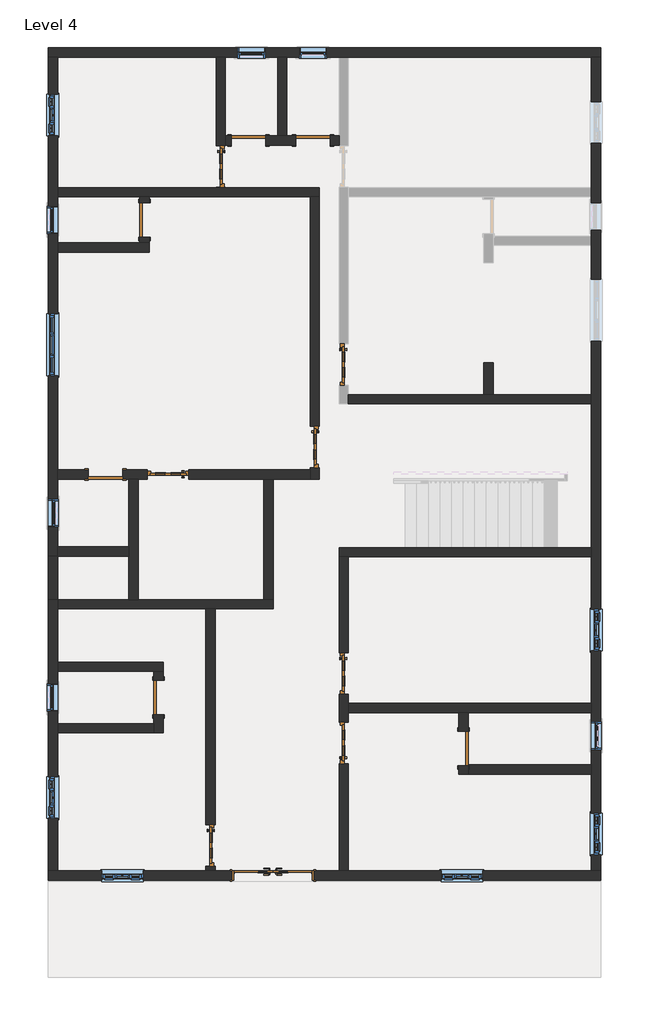
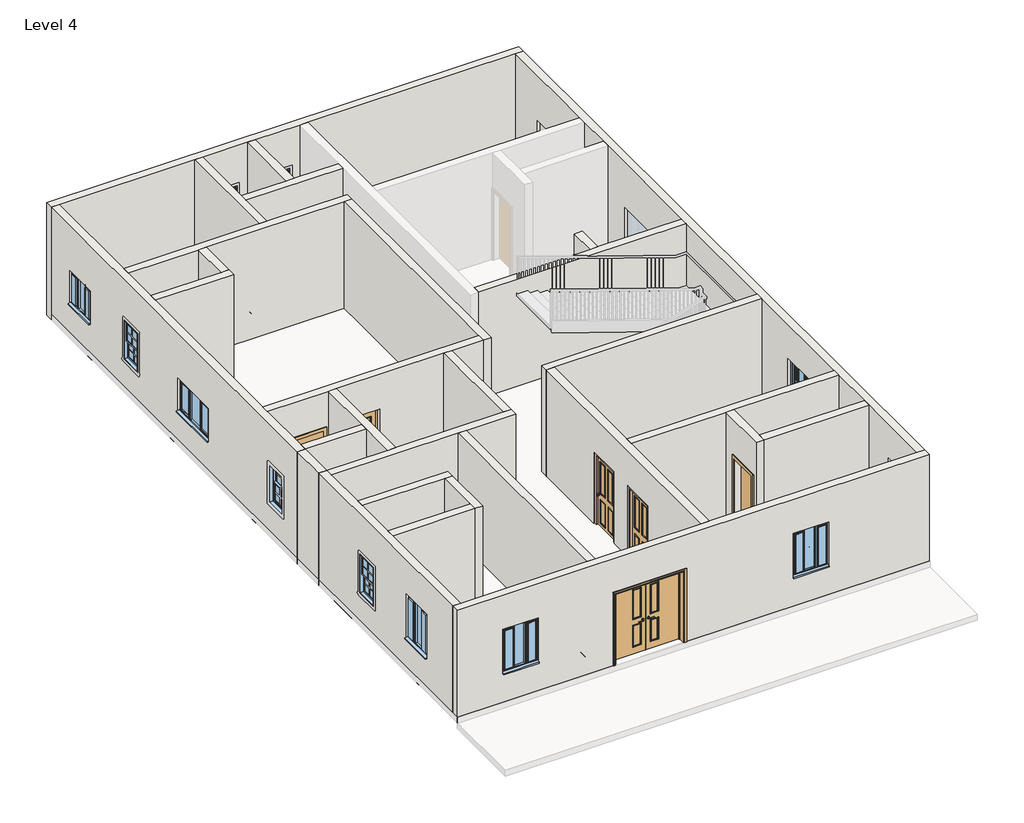
# One storey, part 1 of 3: 29 walls, 14 doors, 13 windows.
# Revit data of these elements (continued)
# Type "Windows_Tpl_Plain : 1360x910mm" (continued)
#   Cavity Closer Depth = 0' - 3.34646"
#   Vis - Cavity Closers = yes
#   Define Thermal Properties by = 1
#   Material Trim = Window Frame
#   Material Glass = Glass
#   Material Frame = Window Frame
#   Wall Closure = (empty or 0)
# Type "Windows_Tpl_w-Glazing_Cross-Bars : 910x1210mm"
#   Type Mark = "25"
#   Operation = "TriplePanelVertical"
#   Construction Type Id = "GSP4R"
#   Manufacturer = "Revit"
#   Keynote = "L10"
#   Analytic Construction = "1/8 in Pilkington single glazing"
#   Wrap Layers (Ext) from Ext = 0' - 4.03543"
#   Wrap Layers (Int) from Ext = 0' - 6.98819"
#   Window Board Projection = 0' - 0.98425"
#   Window Board Extension = 0' - 0.98425"
#   Visual Light Transmittance = 0.9
#   Solar Heat Gain Coefficient = 0.78
#   Rough Width = 2' - 11.82677"
#   Rough Height = 3' - 11.6378"
#   Height = 3' - 11.6378"
#   Width = 2' - 11.82677"
#   Heat Transfer Coefficient (U) = 0.6496 BTU/(h·ft²·°F)
#   Glazing Thickness = 0' - 0.94488"
#   Glazing Bar Thickness = 0' - 0.7874"
#   FrameOffset - External = 0' - 1.9685"
#   Frame Depth = 0' - 2.55906"
#   Default Head Height = 6' - 11.07087"
#   Cill Depth = 0' - 3.44488"
#   Cavity Closer Width = 0' - 1.9685"
#   Cavity Closer Offset from Ext = 0' - 4.03543"
#   Cavity Closer Depth = 0' - 3.34646"
#   Vis - Glazing Bars = yes
#   Vis - Cavity Closers = yes
#   Define Thermal Properties by = 1
#   Material Trim = Window Frame
#   Material Glazing Bars = Window Frame
#   Material Glass = Glass
#   Material Frame = Window Frame
#   Wall Closure = (empty or 0)
# Type "Windows_Tpl_w-Glazing_Cross-Bars : 910x910mm"
#   Type Mark = "24"
#   Operation = "TriplePanelVertical"
#   Construction Type Id = "GSP4R"
#   Manufacturer = "Revit"
#   Keynote = "L10"
#   Analytic Construction = "1/8 in Pilkington single glazing"
#   Wrap Layers (Ext) from Ext = 0' - 4.03543"
#   Wrap Layers (Int) from Ext = 0' - 6.98819"
#   Window Board Projection = 0' - 0.98425"
#   Window Board Extension = 0' - 0.98425"
#   Visual Light Transmittance = 0.9
#   Solar Heat Gain Coefficient = 0.78
#   Rough Width = 2' - 11.82677"
#   Rough Height = 2' - 11.82677"
#   Height = 2' - 11.82677"
#   Width = 2' - 11.82677"
#   Heat Transfer Coefficient (U) = 0.6496 BTU/(h·ft²·°F)
#   Glazing Thickness = 0' - 0.94488"
#   Glazing Bar Thickness = 0' - 0.7874"
#   FrameOffset - External = 0' - 1.9685"
#   Frame Depth = 0' - 2.55906"
#   Default Head Height = 6' - 11.07087"
#   Cill Depth = 0' - 3.44488"
#   Cavity Closer Width = 0' - 1.9685"
#   Cavity Closer Offset from Ext = 0' - 4.03543"
#   Cavity Closer Depth = 0' - 3.34646"
#   Vis - Glazing Bars = yes
#   Vis - Cavity Closers = yes
#   Define Thermal Properties by = 1
#   Material Trim = Window Frame
#   Material Glazing Bars = Window Frame
#   Material Glass = Glass
#   Material Frame = Window Frame
#   Wall Closure = (empty or 0)
# Elements 1, 2, 3, 4, 5, 6, 7 (IfcDoor, "Doors_ExtSgl_2 : 2'x7\"")
#   Phase Created = New Construction
#   Materials on its faces: "Door - Panel", "Door - Handle", "Door - Frame/Mullion", "Door - Glazing"
# Element 8 (IfcDoor, "Doors_IntDbl_3 : 1810x2110mm")
#   Phase Created = New Construction
#   Materials on its faces: "Door - Panel", "Door - Handle", "Door - Architrave", "Door - Frame/Mullion", "Door - Glazing"
# Elements 9, 10, 11, 12, 13, 14 (IfcDoor, "Single-Flush : 30\" x 80\"")
#   Phase Created = New Construction
#   Materials on its faces: "Door - Frame", "Door - Panel"
# Elements 15, 16, 17, 18, 19, 20, 21, 22, 23, 24, 25, 26, 27, 28, 29, 30, 31, 32, 34, 35, 36, 37 (IfcWall, "Generic - 4.5\" p")
#   Top Offset = 0' - 0"
#   Base Offset = 0' - 0"
#   Unconnected Height = 10' - 0"
#   wall height = 10' - 0"
#   Phase Created = New Construction
#   Base Constraint = Level 4
#   Materials on its faces: "Default Wall"
# Elements 33, 38 (IfcWall, "Generic - 4.5\" p")
#   Top Offset = 0' - 0"
#   Base Offset = 0' - 0"
#   Unconnected Height = 10' - 0"
#   wall height = 10' - 0"
#   Phase Created = New Construction
#   Base Constraint = Level 4
#   Materials on its faces: "Default Wall", "Door - Panel"
# Elements 39, 41, 42, 43 (IfcWall, "Generic - 9\" w")
#   Top Offset = 0' - 0"
#   Base Offset = 0' - 0"
#   Unconnected Height = 10' - 0"
#   wall height = 10' - 0"
#   Phase Created = New Construction
#   Base Constraint = Level 4
#   Materials on its faces: "Default Wall", "Door - Panel"
# Element 40 (IfcWall, "Generic - 9\" w")
#   Top Offset = 0' - 0"
#   Base Offset = 0' - 0"
#   Unconnected Height = 10' - 0"
#   wall height = 10' - 0"
#   Phase Created = New Construction
#   Base Constraint = Level 4
#   Materials on its faces: "Default Wall", "Door - Panel", "Default Mass Interior Wall"
# Element 44 (IfcWindow, "Window-Double-Hung : 24\" x 42\"")
#   Mark = "42"
#   Window Inset = 0' - 0"
#   Interior Wall Closure = 0' - 1 1/2"
#   Frame Extension = 0' - 1 1/4"
#   Exterior Wall Closure = 0' - 0 1/2"
#   Interior Trim Visibility = yes
#   Indicator Visibility = yes
#   Exterior Trim Visibility = yes
#   Phase Created = New Construction
#   Materials on its faces: "Wood - Stained", "Glass", "Clad - White"
# Element 45 (IfcWindow, "Window-Double-Hung : 24\" x 42\"")
#   Mark = "43"
#   Window Inset = 0' - 0"
#   Interior Wall Closure = 0' - 1 1/2"
#   Frame Extension = 0' - 1 1/4"
#   Exterior Wall Closure = 0' - 0 1/2"
#   Interior Trim Visibility = yes
#   Indicator Visibility = yes
#   Exterior Trim Visibility = yes
#   Phase Created = New Construction
#   Materials on its faces: "Wood - Stained", "Glass", "Clad - White"
# Element 46 (IfcWindow, "Window-Double-Hung : 24\" x 42\"")
#   Mark = "44"
#   Window Inset = 0' - 0"
#   Interior Wall Closure = 0' - 1 1/2"
#   Frame Extension = 0' - 1 1/4"
#   Exterior Wall Closure = 0' - 0 1/2"
#   Interior Trim Visibility = yes
#   Indicator Visibility = yes
#   Exterior Trim Visibility = yes
#   Phase Created = New Construction
#   Materials on its faces: "Wood - Stained", "Glass", "Clad - White"
# Element 47 (IfcWindow, "Window-Double-Hung : 24\" x 42\"")
#   Mark = "46"
#   Window Inset = 0' - 0"
#   Interior Wall Closure = 0' - 1 1/2"
#   Frame Extension = 0' - 1 1/4"
#   Exterior Wall Closure = 0' - 0 1/2"
#   Interior Trim Visibility = yes
#   Indicator Visibility = yes
#   Exterior Trim Visibility = yes
#   Phase Created = New Construction
#   Materials on its faces: "Wood - Stained", "Glass", "Clad - White"
# Element 48 (IfcWindow, "Window-Double-Hung : 24\" x 42\"")
#   Mark = "47"
#   Window Inset = 0' - 0"
#   Interior Wall Closure = 0' - 1 1/2"
#   Frame Extension = 0' - 1 1/4"
#   Exterior Wall Closure = 0' - 0 1/2"
#   Interior Trim Visibility = yes
#   Indicator Visibility = yes
#   Exterior Trim Visibility = yes
#   Phase Created = New Construction
#   Materials on its faces: "Wood - Stained", "Glass", "Clad - White"
# Element 49 (IfcWindow, "Window-Double-Hung : 24\" x 42\"")
#   Mark = "48"
#   Window Inset = 0' - 0"
#   Interior Wall Closure = 0' - 1 1/2"
#   Frame Extension = 0' - 1 1/4"
#   Exterior Wall Closure = 0' - 0 1/2"
#   Interior Trim Visibility = yes
#   Indicator Visibility = yes
#   Exterior Trim Visibility = yes
#   Phase Created = New Construction
#   Materials on its faces: "Wood - Stained", "Glass", "Clad - White"
# Element 50 (IfcWindow, "Windows_Tpl_Plain : 1360x910mm")
#   Mark = "39"
#   Phase Created = New Construction
#   Materials on its faces: "Window Frame", "Glass"
# Element 51 (IfcWindow, "Windows_Tpl_w-Glazing_Cross-Bars : 910x1210mm")
#   Mark = "33"
#   Phase Created = New Construction
#   Materials on its faces: "Window Frame", "Glass"
# Element 52 (IfcWindow, "Windows_Tpl_w-Glazing_Cross-Bars : 910x1210mm")
#   Mark = "34"
#   Phase Created = New Construction
#   Materials on its faces: "Window Frame", "Glass"
# Element 53 (IfcWindow, "Windows_Tpl_w-Glazing_Cross-Bars : 910x1210mm")
#   Mark = "35"
#   Phase Created = New Construction
#   Materials on its faces: "Window Frame", "Glass"
# Element 54 (IfcWindow, "Windows_Tpl_w-Glazing_Cross-Bars : 910x1210mm")
#   Mark = "36"
#   Phase Created = New Construction
#   Materials on its faces: "Window Frame", "Glass"
# Element 55 (IfcWindow, "Windows_Tpl_w-Glazing_Cross-Bars : 910x1210mm")
#   Mark = "37"
#   Phase Created = New Construction
#   Materials on its faces: "Window Frame", "Glass"
# Element 56 (IfcWindow, "Windows_Tpl_w-Glazing_Cross-Bars : 910x910mm")
#   Mark = "40"
#   Phase Created = New Construction
#   Materials on its faces: "Window Frame", "Glass"
# Materials
#   "Door - Glazing": colour RGB 0 0 255, transparency 0.75
#   "Door - Panel": class "Wood", colour RGB 210 159 95, transparency 0, Cost = 0
#   "Door - Frame/Mullion": class "Wood", colour RGB 212 179 113, transparency 0
#   "Door - Handle": colour RGB 246 240 166, transparency 0
#   "Door - Architrave": class "Wood", colour RGB 154 90 5, transparency 0
#   "Door - Frame": colour RGB 118 70 51, transparency 0, Cost = 0
#   "Wood - Stained": class "Wood", colour RGB 224 178 126, transparency 0, Cost = 0
#   "Clad - White": class "Wood", colour RGB 242 242 238, transparency 0, Cost = 0
#   "Glass": class "Glass", colour RGB 0 128 192, transparency 0.75, Description = "Soda Lime Glass", Cost = 0
#   "Window Frame": colour RGB 249 249 249, transparency 0
#   "Default Wall": colour RGB 128 128 128, transparency 0, Cost = 0
#   "Default Mass Interior Wall": class "Generic", colour RGB 195 229 126, transparency 0, Cost = 0
